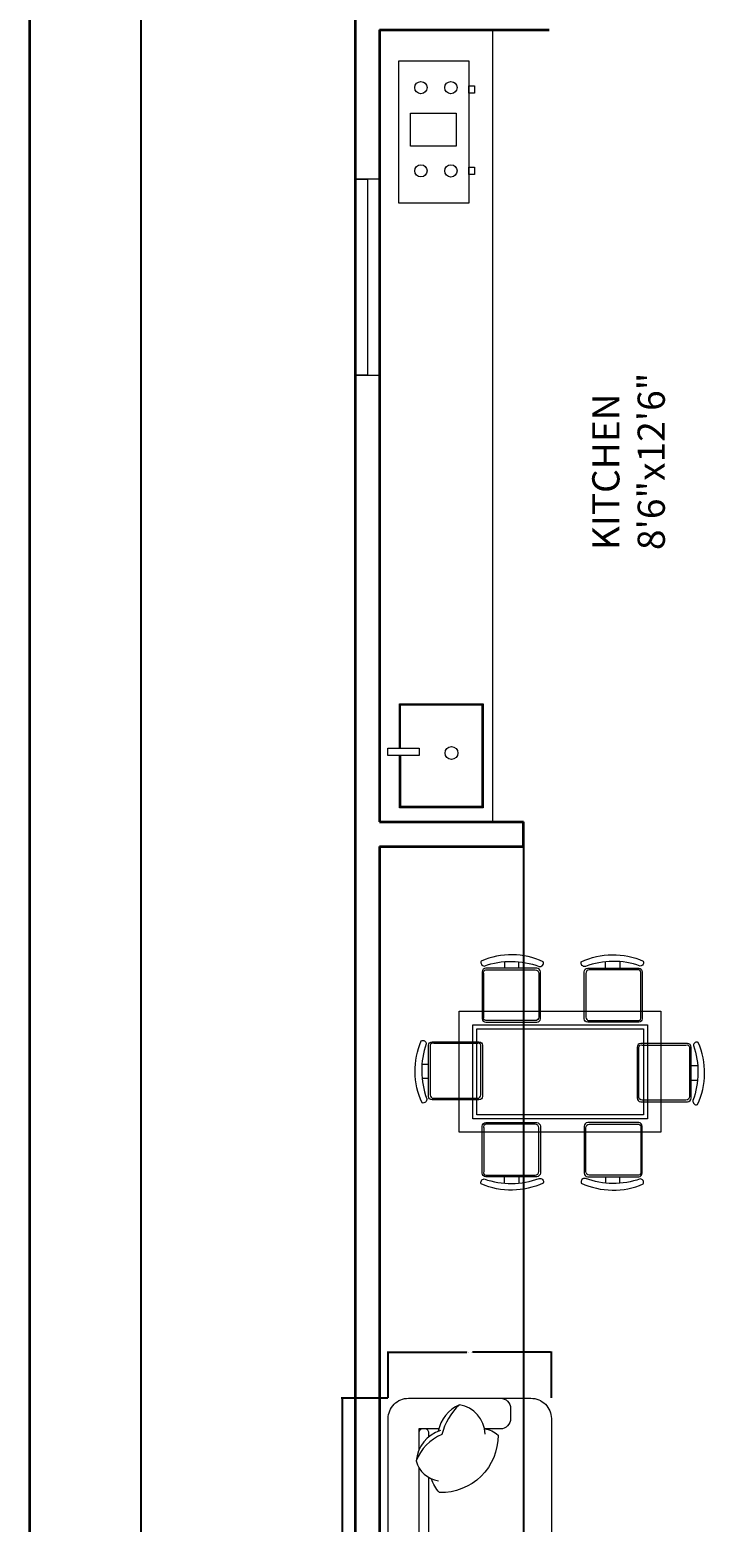
# Model space of a CAD drawing. Units: inches. Extents: x 1734 to 2405, y 1500 to 2491.
# Tile 11 of 14: x 1734 to 1862, y 2078 to 2352. Entities that reach past the tile are written whole.
import ezdxf

# ---------------------------------------------------------------- set-up
doc = ezdxf.new("R2010")
doc.units = ezdxf.units.IN
for name, color, linetype, lineweight in [('A-ANNO-DIMS', 2, 'Continuous', 18), ('A-ANNO-TTLB', 7, 'Continuous', 35), ('A-AREA-IDEN', 7, 'Continuous', 18), ('A-EQPM', 8, 'Continuous', 18), ('A-FLOR-CASE', 9, 'Continuous', 18), ('A-FLOR-FIXT', 9, 'Continuous', 18), ('A-FURN', 8, 'Continuous', 13), ('A-GLAZ', 4, 'Continuous', 18), ('A-WALL', 7, 'Continuous', 35)]:
    doc.layers.add(name, color=color, linetype=linetype, lineweight=lineweight)
doc.styles.get("Standard").update_dxf_attribs({"font": 'arial.ttf'})
doc.dimstyles.get("Standard").update_dxf_attribs({"dimtxt": 0.18, "dimasz": 0.18, "dimexe": 0.18, "dimexo": 0.0625, "dimgap": 0.09, "dimtad": 0, "dimtih": 1, "dimtoh": 1, "dimdec": 4, "dimzin": 0, "dimdsep": 46, "dimtxsty": 'Standard', "dimcen": 0.09, "dimadec": 0, "dimazin": 0, "dimtfac": 1, "dimtdec": 4, "dimtofl": 0, "dimtmove": 0, "dimatfit": 3, "dimfxl": 1, "dimtolj": 1, "dimtzin": 0, "dimarcsym": 0})

# ---------------------------------------------------------------- blocks, each defined once
blk = doc.blocks.new('SOFA-COMPACT')
at = {"ltscale": 0.03}
blk.add_lwpolyline([(29.99, 29.99, -0.414214), (28.12, 28.12, -0.414214), (29.99, 26.24), (29.99, 3.75, -0.414214), (26.24, 0), (3.75, 0, -0.414214), (0, 3.75), (0, 52.49, -0.414214), (3.75, 56.24), (26.24, 56.24, -0.414214), (29.99, 52.49), (29.99, 29.99, -0.414214), (28.12, 28.12, -0.414214), (29.99, 26.24)], format="xyb", dxfattribs=at)
for points in [[(13.1, 55.04, 0.14773), (9.88, 49.56, 0.213343), (5.16, 44.73, 0.178662)], [(17.83, 49.67, 0.356772), (13.1, 55.04, 0.249542), (9.21, 50.18, -9.61688)], [(20.62, 56.24, -0.414214), (22.49, 54.36), (22.49, 52.49, -0.414214), (20.62, 50.61), (17.72, 50.61)], [(9.63, 50.32, 0.306663), (5.16, 44.73, 0.30633), (9.24, 41.08, -0.872847)], [(7.5, 49.18), (7.5, 49.86, 0.414214), (6.75, 50.61), (6.37, 50.61, 0.414214), (5.62, 49.86)], [(5.62, 49.86), (5.62, 46.67, 0.414214)], [(17.71, 50.62, -0.165541), (20.19, 49.46, -0.425989), (9.45, 38.93, -0.121523), (7.97, 41.43, 7.115464)], [(5.62, 43.55), (5.62, 28.87, 0.414214), (6.37, 28.12), (6.75, 28.12, 0.414214), (7.5, 28.87), (7.5, 41.66, 0.414214)], [(5.62, 22.78), (5.62, 27.37, -0.414214), (6.37, 28.12), (6.75, 28.12, -0.414214), (7.5, 27.37), (7.5, 24.67, -0.414214)], [(7.5, 29.99, 0.414214), (9.37, 28.12)], [(7.5, 29.99, 0.414214), (9.37, 28.12), (28.12, 28.12, 0.414214)], [(7.5, 26.24, -0.414214), (9.37, 28.12)], [(7.5, 26.24, -0.414214), (9.37, 28.12), (28.12, 28.12, -0.414214)], [(9.63, 16.01, -0.306663), (5.16, 21.6, -0.30633), (9.24, 25.26, 0.872847)], [(17.71, 15.72, 0.165541), (20.19, 16.88, 0.425989), (9.45, 27.4, 0.121523), (7.97, 24.91, -7.115464)], [(13.1, 11.29, -0.14773), (9.88, 16.77, -0.213343), (5.16, 21.6, -0.178662)], [(5.62, 12.69), (5.62, 19.67, -0.414214)], [(7.5, 17.15), (7.5, 14.57, -0.414214)], [(17.83, 16.66, -0.356772), (13.1, 11.29, -0.249542), (9.21, 16.16, 9.61688)], [(9.63, 5.91, -0.306663), (5.16, 11.51, -0.30633), (9.24, 15.16, 0.872847)], [(8.71, 16.38, 0.071865), (7.97, 14.81, -7.115464)], [(17.71, 5.62, 0.165541), (20.19, 6.78, 0.200231), (17.17, 14.22, 0.121523)], [(13.1, 1.19, -0.14773), (9.88, 6.67, -0.213343), (5.16, 11.51, -0.178662)], [(5.62, 6.37), (5.62, 9.57, -0.414214)], [(5.62, 9.57), (5.62, 5.62), (9.31, 5.62, -0.414214)], [(7.5, 7.05), (7.5, 6.37, -0.414214), (6.75, 5.62), (6.37, 5.62, -0.414214), (5.62, 6.37)], [(17.83, 6.56, -0.356772), (13.1, 1.19, -0.249542), (9.21, 6.06, 9.61688)], [(17.72, 5.62), (20.62, 5.62, -0.414214), (22.49, 3.75), (22.49, 1.87, -0.414214), (20.62, 0)]]:
    blk.add_lwpolyline(points, format="xyb")
for points in [[(9.31, 50.61), (5.62, 50.61), (5.62, 46.67)], [(5.62, 43.55), (5.62, 22.78)], [(5.62, 19.67), (5.62, 12.69)]]:
    blk.add_lwpolyline(points)
blk.add_lwpolyline([(5.62, 28.87), (5.62, 27.37, -0.414214), (6.37, 28.12), (6.75, 28.12, -0.414214), (7.5, 27.37), (7.5, 28.87, -0.414214), (6.75, 28.12), (6.37, 28.12, -0.414214)], format="xyb", close=True)
blk = doc.blocks.new('*D12')
at = {"layer": 'A-ANNO-DIMS', "color": 0, "lineweight": -2, "transparency": 16777216}
for p, q in [((1799.89, 2100.96), (1791.34, 2100.96)), ((1791.52, 2100.78), (1791.52, 2073.03)), ((1791.52, 2044.91), (1791.52, 2072.66)), ((1799.89, 2044.73), (1791.34, 2044.73))]:
    blk.add_line(p, q, dxfattribs=at)
at = {"layer": 'A-ANNO-DIMS', "color": 0, "transparency": 16777216}
for points in [[(1791.49, 2100.78), (1791.55, 2100.78), (1791.52, 2100.96)], [(1791.49, 2044.91), (1791.55, 2044.91), (1791.52, 2044.73)]]:
    blk.add_solid(points, dxfattribs=at)
at = {"layer": 'Defpoints', "color": 0, "transparency": 16777216}
for p in [(1791.52, 2100.96), (1799.96, 2100.96), (1799.96, 2044.73)]:
    blk.add_point(p, dxfattribs=at)
at = {"layer": 'A-ANNO-DIMS', "color": 0, "transparency": 16777216, "insert": (1791.52, 2072.84), "char_height": 0.18, "attachment_point": 5}
blk.add_mtext('\\A1;SOFA 56 TYP.', dxfattribs=at)
blk = doc.blocks.new('*D13')
at = {"layer": 'A-ANNO-DIMS', "color": 0, "lineweight": -2, "transparency": 16777216}
for p, q in [((1799.96, 2101.02), (1799.96, 2109.58)), ((1800.14, 2109.4), (1814.42, 2109.4)), ((1829.77, 2109.4), (1815.48, 2109.4)), ((1829.95, 2101.02), (1829.95, 2109.58))]:
    blk.add_line(p, q, dxfattribs=at)
at = {"layer": 'A-ANNO-DIMS', "color": 0, "transparency": 16777216}
for points in [[(1800.14, 2109.43), (1800.14, 2109.37), (1799.96, 2109.4)], [(1829.77, 2109.43), (1829.77, 2109.37), (1829.95, 2109.4)]]:
    blk.add_solid(points, dxfattribs=at)
at = {"layer": 'Defpoints', "color": 0, "transparency": 16777216}
for p in [(1829.95, 2109.4), (1799.96, 2100.96), (1829.95, 2100.96)]:
    blk.add_point(p, dxfattribs=at)
at = {"layer": 'A-ANNO-DIMS', "color": 0, "transparency": 16777216, "insert": (1814.95, 2109.4), "char_height": 0.18, "attachment_point": 5}
blk.add_mtext('\\A1;30 TYP.', dxfattribs=at)
blk = doc.blocks.new('*D23')
at = {"layer": 'A-ANNO-DIMS', "color": 0, "lineweight": -2, "transparency": 16777216}
for p, q in [((1793.83, 2425.82), (1754.36, 2425.82)), ((1754.54, 2425.64), (1754.54, 2068.48)), ((1754.54, 1710.95), (1754.54, 2068.11)), ((1793.83, 1710.77), (1754.36, 1710.77))]:
    blk.add_line(p, q, dxfattribs=at)
at = {"layer": 'A-ANNO-DIMS', "color": 0, "transparency": 16777216}
for points in [[(1754.51, 2425.64), (1754.57, 2425.64), (1754.54, 2425.82)], [(1754.51, 1710.95), (1754.57, 1710.95), (1754.54, 1710.77)]]:
    blk.add_solid(points, dxfattribs=at)
at = {"layer": 'Defpoints', "color": 0, "transparency": 16777216}
for p in [(1754.54, 2425.82), (1793.89, 2425.82), (1793.89, 1710.77)]:
    blk.add_point(p, dxfattribs=at)
at = {"layer": 'A-ANNO-DIMS', "color": 0, "transparency": 16777216, "insert": (1754.54, 2068.3), "char_height": 0.18, "attachment_point": 5}
blk.add_mtext('\\A1;715', dxfattribs=at)
blk = doc.blocks.new('*D32')
at = {"layer": 'A-ANNO-DIMS', "color": 0, "lineweight": -2, "transparency": 16777216}
for p, q in [((1798.39, 2202.26), (1798.39, 1615.47)), ((1824.83, 2202.26), (1824.83, 1615.47)), ((1798.57, 1615.65), (1811.22, 1615.65)), ((1824.65, 1615.65), (1812.01, 1615.65))]:
    blk.add_line(p, q, dxfattribs=at)
at = {"layer": 'A-ANNO-DIMS', "color": 0, "transparency": 16777216}
for points in [[(1798.57, 1615.68), (1798.57, 1615.62), (1798.39, 1615.65)], [(1824.65, 1615.68), (1824.65, 1615.62), (1824.83, 1615.65)]]:
    blk.add_solid(points, dxfattribs=at)
at = {"layer": 'Defpoints', "color": 0, "transparency": 16777216}
for p in [(1798.39, 2202.32), (1824.83, 2202.32), (1824.83, 1615.65)]:
    blk.add_point(p, dxfattribs=at)
at = {"layer": 'A-ANNO-DIMS', "color": 0, "transparency": 16777216, "insert": (1811.61, 1615.65), "char_height": 0.18, "attachment_point": 5}
blk.add_mtext('\\A1;26.44', dxfattribs=at)
blk = doc.blocks.new('*D33')
at = {"layer": 'A-ANNO-DIMS', "color": 0, "lineweight": -2, "transparency": 16777216}
for p, q in [((1824.83, 2202.26), (1824.83, 1615.47)), ((1874.68, 2202.26), (1874.68, 1615.47)), ((1825.01, 1615.65), (1849.36, 1615.65)), ((1874.5, 1615.65), (1850.15, 1615.65))]:
    blk.add_line(p, q, dxfattribs=at)
at = {"layer": 'A-ANNO-DIMS', "color": 0, "transparency": 16777216}
for points in [[(1825.01, 1615.68), (1825.01, 1615.62), (1824.83, 1615.65)], [(1874.5, 1615.68), (1874.5, 1615.62), (1874.68, 1615.65)]]:
    blk.add_solid(points, dxfattribs=at)
at = {"layer": 'Defpoints', "color": 0, "transparency": 16777216}
for p in [(1824.83, 2202.32), (1874.68, 2202.32), (1874.68, 1615.65)]:
    blk.add_point(p, dxfattribs=at)
at = {"layer": 'A-ANNO-DIMS', "color": 0, "transparency": 16777216, "insert": (1849.76, 1615.65), "char_height": 0.18, "attachment_point": 5}
blk.add_mtext('\\A1;49.84', dxfattribs=at)

msp = doc.modelspace()

# ---------------------------------------------------------------- linework, layer by layer
at = {"layer": 'A-ANNO-TTLB'}
msp.add_lwpolyline([(1734.1307, 2491.1293), (2404.5589, 2491.1293), (2404.5589, 1500.293), (1734.1307, 1500.293)], close=True, dxfattribs=at)
at = {"layer": 'A-EQPM'}
for points in [[(1801.9497, 2346.6244), (1814.7817, 2346.6244), (1814.7817, 2320.5066), (1801.9497, 2320.5066)], [(1814.7817, 2342.041), (1815.82, 2342.041), (1815.82, 2340.6935), (1814.7817, 2340.6935)], [(1804.0877, 2336.9934), (1812.4457, 2336.9934), (1812.4457, 2330.9836), (1804.0877, 2330.9836)], [(1814.7817, 2327.0852), (1815.82, 2327.0852), (1815.82, 2325.7377), (1814.7817, 2325.7377)]]:
    msp.add_lwpolyline(points, close=True, dxfattribs=at)
for centre in [(1805.9861, 2341.7074), (1811.4968, 2341.7074), (1805.9861, 2326.4232), (1811.4968, 2326.4106)]:
    msp.add_circle(centre, 1.1254, dxfattribs=at)
at = {"layer": 'A-FLOR-CASE'}
msp.add_line((1819.2014, 2206.8246), (1819.2014, 2352.3246), dxfattribs=at)
at = {"layer": 'A-FLOR-FIXT'}
for p, q in [((1802.23, 2220.3738), (1802.23, 2228.5425)), ((1802.23, 2228.5425), (1802.23, 2228.4132)), ((1802.23, 2228.4132), (1802.23, 2228.3479)), ((1802.23, 2228.3479), (1817.4383, 2228.3479)), ((1817.4383, 2228.3479), (1817.1655, 2228.3479)), ((1817.1655, 2228.3479), (1817.1655, 2209.4249)), ((1802.0555, 2220.3738), (1802.23, 2220.3738)), ((1802.265, 2209.6534), (1802.265, 2219.0009)), ((1817.1655, 2209.6534), (1802.0555, 2209.6534)), ((1802.0555, 2209.6534), (1802.265, 2209.6534)), ((1817.1655, 2209.4249), (1817.1655, 2209.6534))]:
    msp.add_line(p, q, dxfattribs=at)
msp.add_lwpolyline([(1802.0555, 2220.3738), (1802.0555, 2228.5425), (1817.4383, 2228.5425), (1817.4383, 2209.4249), (1802.0555, 2209.4249), (1802.0555, 2219.0009)], dxfattribs=at)
msp.add_lwpolyline([(1799.9266, 2220.3738), (1805.6608, 2220.3738), (1805.6608, 2219.0009), (1799.9266, 2219.0009)], close=True, dxfattribs=at)
msp.add_circle((1811.5924, 2219.4842), 1.189, dxfattribs=at)
at = {"layer": 'A-FURN'}
for points in [[(1817.6044, 2180.3628, -0.17580919), (1827.6967, 2180.2863, 0.57839206), (1828.4613, 2181.127, 0.21452438), (1817.0692, 2181.2799, 0.55201397), (1817.6044, 2180.3628, -0.06507904)], [(1817.6044, 2180.3624, -0.17580919), (1827.6967, 2180.286, 0.57839206), (1828.4613, 2181.1267, 0.21452438), (1817.0692, 2181.2795, 0.55201397), (1817.6044, 2180.3624, -0.06507904)], [(1836.1931, 2180.2863, -0.57839206), (1835.4286, 2181.127, -0.21452438), (1846.8207, 2181.2799, -0.55201397), (1846.2855, 2180.3628, 0.1758092), (1836.1932, 2180.2863)], [(1836.1932, 2180.286, -0.57839206), (1835.4286, 2181.1267, -0.21452438), (1846.8207, 2181.2795, -0.55201397), (1846.2855, 2180.3624, 0.1758092), (1836.1932, 2180.286)], [(1827.2685, 2179.9577), (1817.8992, 2179.9577, 0.41421356), (1817.2437, 2179.3022), (1817.2437, 2170.6873, 0.41421356), (1817.8992, 2170.0318), (1827.2685, 2170.0318, 0.41421356), (1827.924, 2170.6873), (1827.924, 2179.3022, 0.41421356), (1827.2685, 2179.9577)], [(1827.2686, 2179.9573), (1817.8992, 2179.9573, 0.41421356), (1817.2437, 2179.3018), (1817.2437, 2170.6869, 0.41421356), (1817.8992, 2170.0314), (1827.2686, 2170.0314, 0.41421356), (1827.924, 2170.6869), (1827.924, 2179.3018, 0.41421356), (1827.2686, 2179.9573)], [(1823.9775, 2179.9577), (1823.9775, 2181.1427, -0.06475861)], [(1823.9776, 2179.9573), (1823.9776, 2181.1423, -0.06475861)], [(1845.9907, 2179.9577, -0.41421356), (1846.6462, 2179.3022), (1846.6462, 2170.6873, -0.41421356), (1845.9907, 2170.0318), (1836.6213, 2170.0318, -0.41421356), (1835.9658, 2170.6873), (1835.9658, 2179.3022, -0.41421356), (1836.6213, 2179.9577), (1845.9907, 2179.9577)], [(1845.9907, 2179.9573, -0.41421356), (1846.6462, 2179.3018), (1846.6462, 2170.6869, -0.41421356), (1845.9907, 2170.0314), (1836.6213, 2170.0314, -0.41421356), (1835.9658, 2170.6869), (1835.9658, 2179.3018, -0.41421356), (1836.6213, 2179.9573), (1845.9907, 2179.9573)], [(1839.9123, 2179.9577), (1839.9123, 2181.1427, 0.06475861)], [(1839.9123, 2179.9573), (1839.9123, 2181.1423, 0.06475861)], [(1807.0459, 2155.9913, -0.57839206), (1806.2052, 2155.2268, -0.21452438), (1806.0523, 2166.6189, -0.55201397), (1806.9694, 2166.0837, 0.17580937), (1807.0459, 2155.9913)], [(1807.0459, 2155.9909, -0.57839206), (1806.2052, 2155.2264, -0.21452438), (1806.0523, 2166.6185, -0.55201397), (1806.9695, 2166.0833, 0.17580937), (1807.0459, 2155.9909)], [(1807.3745, 2165.7889, -0.41421356), (1808.03, 2166.4444), (1816.645, 2166.4444, -0.41421356), (1817.3004, 2165.7889), (1817.3004, 2156.4195, -0.41421356), (1816.645, 2155.764), (1808.03, 2155.764, -0.41421356), (1807.3745, 2156.4195), (1807.3745, 2165.7889)], [(1807.3745, 2165.7885, -0.41421356), (1808.03, 2166.444), (1816.645, 2166.444, -0.41421356), (1817.3005, 2165.7885), (1817.3005, 2156.4191, -0.41421356), (1816.645, 2155.7636), (1808.03, 2155.7636, -0.41421356), (1807.3745, 2156.4191), (1807.3745, 2165.7885)], [(1855.6224, 2165.468, 0.41421356), (1854.9669, 2166.1235), (1846.3519, 2166.1235, 0.41421356), (1845.6965, 2165.468), (1845.6965, 2156.0986, 0.41421356), (1846.3519, 2155.4431), (1854.9669, 2155.4431, 0.41421356), (1855.6224, 2156.0986), (1855.6224, 2165.468)], [(1855.6224, 2165.4676, 0.41421356), (1854.9669, 2166.1231), (1846.352, 2166.1231, 0.41421356), (1845.6965, 2165.4676), (1845.6965, 2156.0982, 0.41421356), (1846.352, 2155.4427), (1854.9669, 2155.4427, 0.41421356), (1855.6224, 2156.0982), (1855.6224, 2165.4676)], [(1856.0275, 2165.7628, -0.17580919), (1855.951, 2155.6705, 0.57839206), (1856.7917, 2154.9059, 0.21452438), (1856.9446, 2166.298, 0.55201397), (1856.0275, 2165.7628, -0.06507904)], [(1856.0275, 2165.7624, -0.17580919), (1855.9511, 2155.6701, 0.57839206), (1856.7918, 2154.9055, 0.21452438), (1856.9446, 2166.2976, 0.55201397), (1856.0275, 2165.7624, -0.06507904)], [(1807.3745, 2159.7105), (1806.1896, 2159.7105, 0.06475861)], [(1807.3745, 2159.7101), (1806.1896, 2159.7101, 0.06475861)], [(1855.6224, 2159.3896), (1856.8073, 2159.3896, -0.06475861)], [(1855.6224, 2159.3892), (1856.8074, 2159.3892, -0.06475861)], [(1827.2685, 2141.6621), (1817.8992, 2141.6621, -0.41421356), (1817.2437, 2142.3176), (1817.2437, 2150.9326, -0.41421356), (1817.8992, 2151.5881), (1827.2685, 2151.5881, -0.41421356), (1827.924, 2150.9326), (1827.924, 2142.3176, -0.41421356), (1827.2685, 2141.6621)], [(1827.2686, 2141.6617), (1817.8992, 2141.6617, -0.41421356), (1817.2437, 2142.3172), (1817.2437, 2150.9322, -0.41421356), (1817.8992, 2151.5877), (1827.2686, 2151.5877, -0.41421356), (1827.924, 2150.9322), (1827.924, 2142.3172, -0.41421356), (1827.2686, 2141.6617)], [(1845.9907, 2141.6621, 0.41421356), (1846.6462, 2142.3176), (1846.6462, 2150.9326, 0.41421356), (1845.9907, 2151.5881), (1836.6213, 2151.5881, 0.41421356), (1835.9658, 2150.9326), (1835.9658, 2142.3176, 0.41421356), (1836.6213, 2141.6621), (1845.9907, 2141.6621)], [(1845.9907, 2141.6617, 0.41421356), (1846.6462, 2142.3172), (1846.6462, 2150.9322, 0.41421356), (1845.9907, 2151.5877), (1836.6213, 2151.5877, 0.41421356), (1835.9658, 2150.9322), (1835.9658, 2142.3172, 0.41421356), (1836.6213, 2141.6617), (1845.9907, 2141.6617)], [(1827.6967, 2141.3335, -0.57839206), (1828.4613, 2140.4928, -0.21452438), (1817.0692, 2140.3399, -0.55201397), (1817.6044, 2141.257, 0.17580929), (1827.6967, 2141.3335)], [(1827.6967, 2141.3331, -0.57839206), (1828.4613, 2140.4924, -0.21452438), (1817.0692, 2140.3395, -0.55201397), (1817.6044, 2141.2567, 0.17580929), (1827.6967, 2141.3331)], [(1823.9775, 2141.6621), (1823.9775, 2140.4772, 0.06475861)], [(1823.9776, 2141.6617), (1823.9776, 2140.4768, 0.06475861)], [(1846.2855, 2141.257, -0.17580928), (1836.1931, 2141.3335, 0.57839206), (1835.4286, 2140.4928, 0.21452438), (1846.8207, 2140.3399, 0.55201397), (1846.2855, 2141.257, -0.06507904)], [(1846.2855, 2141.2567, -0.17580928), (1836.1932, 2141.3331, 0.57839206), (1835.4286, 2140.4924, 0.21452438), (1846.8207, 2140.3395, 0.55201397), (1846.2855, 2141.2567, -0.06507904)], [(1839.9123, 2141.6621), (1839.9123, 2140.4772, -0.06475861)], [(1839.9123, 2141.6617), (1839.9123, 2140.4768, -0.06475861)]]:
    msp.add_lwpolyline(points, format="xyb", dxfattribs=at)
for points in [[(1817.9031, 2179.6624), (1826.9732, 2179.6624, -0.41421356), (1827.6287, 2179.0069), (1827.6287, 2170.9826, -0.41421356), (1826.9732, 2170.3271), (1817.9031, 2170.3271, -0.51206948), (1817.539, 2170.9826), (1817.539, 2179.0069, -0.51206948)], [(1817.9032, 2179.662), (1826.9732, 2179.662, -0.41421356), (1827.6287, 2179.0065), (1827.6287, 2170.9822, -0.41421356), (1826.9732, 2170.3267), (1817.9032, 2170.3267, -0.51206948), (1817.539, 2170.9822), (1817.539, 2179.0065, -0.51206948)], [(1845.9867, 2179.6624), (1836.9166, 2179.6624, 0.41421356), (1836.2611, 2179.0069), (1836.2611, 2170.9826, 0.41421356), (1836.9166, 2170.3271), (1845.9867, 2170.3271, 0.51206948), (1846.3509, 2170.9826), (1846.3509, 2179.0069, 0.51206948)], [(1845.9867, 2179.662), (1836.9166, 2179.662, 0.41421356), (1836.2612, 2179.0065), (1836.2612, 2170.9822, 0.41421356), (1836.9166, 2170.3267), (1845.9867, 2170.3267, 0.51206948), (1846.3509, 2170.9822), (1846.3509, 2179.0065, 0.51206948)], [(1807.6698, 2165.7849), (1807.6698, 2156.7148, 0.41421356), (1808.3253, 2156.0593), (1816.3497, 2156.0593, 0.41421356), (1817.0051, 2156.7148), (1817.0051, 2165.7849, 0.51206948), (1816.3497, 2166.1491), (1808.3253, 2166.1491, 0.51206948)], [(1807.6698, 2165.7845), (1807.6698, 2156.7144, 0.41421356), (1808.3253, 2156.0589), (1816.3497, 2156.0589, 0.41421356), (1817.0052, 2156.7144), (1817.0052, 2165.7845, 0.51206948), (1816.3497, 2166.1487), (1808.3253, 2166.1487, 0.51206948)], [(1855.3271, 2165.464), (1855.3271, 2156.3939, -0.41421356), (1854.6716, 2155.7384), (1846.6473, 2155.7384, -0.41421356), (1845.9918, 2156.3939), (1845.9918, 2165.464, -0.51206948), (1846.6473, 2165.8282), (1854.6716, 2165.8282, -0.51206948)], [(1855.3271, 2165.4636), (1855.3271, 2156.3935, -0.41421356), (1854.6716, 2155.738), (1846.6473, 2155.738, -0.41421356), (1845.9918, 2156.3935), (1845.9918, 2165.4636, -0.51206948), (1846.6473, 2165.8278), (1854.6716, 2165.8278, -0.51206948)], [(1817.9031, 2141.9574), (1826.9732, 2141.9574, 0.41421356), (1827.6287, 2142.6129), (1827.6287, 2150.6373, 0.41421356), (1826.9732, 2151.2927), (1817.9031, 2151.2927, 0.51206948), (1817.539, 2150.6373), (1817.539, 2142.6129, 0.51206948)], [(1817.9032, 2141.957), (1826.9732, 2141.957, 0.41421356), (1827.6287, 2142.6125), (1827.6287, 2150.6369, 0.41421356), (1826.9732, 2151.2924), (1817.9032, 2151.2924, 0.51206948), (1817.539, 2150.6369), (1817.539, 2142.6125, 0.51206948)], [(1845.9867, 2141.9574), (1836.9166, 2141.9574, -0.41421356), (1836.2611, 2142.6129), (1836.2611, 2150.6373, -0.41421356), (1836.9166, 2151.2927), (1845.9867, 2151.2927, -0.51206948), (1846.3509, 2150.6373), (1846.3509, 2142.6129, -0.51206948)], [(1845.9867, 2141.957), (1836.9166, 2141.957, -0.41421356), (1836.2612, 2142.6125), (1836.2612, 2150.6369, -0.41421356), (1836.9166, 2151.2924), (1845.9867, 2151.2924, -0.51206948), (1846.3509, 2150.6369), (1846.3509, 2142.6125, -0.51206948)]]:
    msp.add_lwpolyline(points, format="xyb", close=True, dxfattribs=at)
for points in [[(1821.3549, 2181.1642), (1821.3549, 2179.9577)], [(1821.3549, 2181.1638), (1821.3549, 2179.9573)], [(1842.5349, 2181.1642), (1842.5349, 2179.9577)], [(1842.535, 2181.1638), (1842.535, 2179.9573)], [(1806.168, 2162.3331), (1807.3745, 2162.3331)], [(1806.168, 2162.3327), (1807.3745, 2162.3327)], [(1856.8289, 2162.0122), (1855.6224, 2162.0122)], [(1856.8289, 2162.0119), (1855.6224, 2162.0119)], [(1821.3549, 2140.4556), (1821.3549, 2141.6621)], [(1821.3549, 2140.4552), (1821.3549, 2141.6617)], [(1842.5349, 2140.4556), (1842.5349, 2141.6621)], [(1842.535, 2140.4552), (1842.535, 2141.6617)]]:
    msp.add_lwpolyline(points, dxfattribs=at)
for points in [[(1813.0212, 2172.045), (1850.0748, 2172.045), (1850.0748, 2149.8129), (1813.0212, 2149.8129)], [(1813.0213, 2172.0446), (1850.0748, 2172.0446), (1850.0748, 2149.8125), (1813.0213, 2149.8125)], [(1815.4915, 2169.5748), (1847.6045, 2169.5748), (1847.6045, 2152.2832), (1815.4915, 2152.2832)], [(1815.4915, 2169.5744), (1847.6046, 2169.5744), (1847.6046, 2152.2828), (1815.4915, 2152.2828)], [(1816.2325, 2168.8337), (1846.8635, 2168.8337), (1846.8635, 2153.0242), (1816.2325, 2153.0242)], [(1816.2326, 2168.8333), (1846.8635, 2168.8333), (1846.8635, 2153.0238), (1816.2326, 2153.0238)]]:
    msp.add_lwpolyline(points, close=True, dxfattribs=at)
at = {"layer": 'A-GLAZ'}
for p, q in [((1798.3942, 2324.9064), (1793.8942, 2324.9064)), ((1793.8942, 2324.9064), (1796.1442, 2324.9064)), ((1796.1442, 2324.9064), (1796.1442, 2288.9064)), ((1796.1442, 2288.9064), (1793.8942, 2288.9064)), ((1793.8942, 2288.9064), (1798.3942, 2288.9064))]:
    msp.add_line(p, q, dxfattribs=at)
at = {"layer": 'A-WALL'}
for p, q in [((1793.8942, 2425.8246), (1793.8942, 1891.8246)), ((1798.3942, 2352.3246), (1829.5495, 2352.3246)), ((1798.3942, 2352.3246), (1798.3942, 2206.8246)), ((1798.3942, 2206.8246), (1824.8343, 2206.8246)), ((1824.8343, 2202.3246), (1824.8343, 2206.8246)), ((1798.3942, 2202.3246), (1824.8343, 2202.3246)), ((1798.3942, 2202.3246), (1798.3942, 1956.3246))]:
    msp.add_line(p, q, dxfattribs=at)

# ---------------------------------------------------------------- block references
at = {"layer": 'A-FURN'}
msp.add_blockref('SOFA-COMPACT', (1799.957, 2044.726), dxfattribs=at)

# ---------------------------------------------------------------- texts
at = {"layer": 'A-AREA-IDEN', "insert": (1837.4539, 2256.766), "char_height": 5, "attachment_point": 1, "rotation": 90}
msp.add_mtext_dynamic_manual_height_columns('KITCHEN\\P8\'6"x12\'6"', width=162.854422, gutter_width=12.5, heights=[0], dxfattribs=at)

# ---------------------------------------------------------------- dimensions: what is measured, and where the dimension line sits
at = {"layer": 'A-ANNO-DIMS'}
dim = msp.add_linear_dim(base=(1754.5442, 2425.8246), p1=(1793.8942, 1710.7667), p2=(1793.8942, 2425.8246), angle=90, dimstyle='Standard', override={"dimdec": 0, "dimlfac": 1, "dimrnd": 0, "dimzin": 0, "dimdsep": 46, "dimlunit": 2}, dxfattribs=at)
dim.commit()
dim.dimension.update_dxf_attribs({"geometry": '*D23', "text_midpoint": (1754.5442, 2068.2956)})
for base, p1, p2, picture, middle in [((1824.8343, 1615.6468), (1798.3942, 2202.3246), (1824.8343, 2202.3246), '*D32', (1811.6142, 1615.6468)), ((1874.676, 1615.6468), (1824.8343, 2202.3246), (1874.676, 2202.3246), '*D33', (1849.7551, 1615.6468))]:
    dim = msp.add_linear_dim(base=base, p1=p1, p2=p2, dimstyle='Standard', override={"dimdec": 2, "dimlfac": 1, "dimrnd": 0, "dimzin": 0, "dimdsep": 46, "dimlunit": 2}, dxfattribs=at)
    dim.commit()
    dim.dimension.update_dxf_attribs({"geometry": picture, "text_midpoint": middle})
dim = msp.add_linear_dim(base=(1829.9488, 2109.3966), p1=(1799.9567, 2100.9613), p2=(1829.9488, 2100.9613), text='<> TYP.', dimstyle='Standard', override={"dimdec": 0, "dimlfac": 1, "dimrnd": 0, "dimzin": 0, "dimdsep": 46, "dimlunit": 2}, dxfattribs=at)
dim.commit()
dim.dimension.update_dxf_attribs({"geometry": '*D13', "text_midpoint": (1814.9528, 2109.3966)})
dim = msp.add_linear_dim(base=(1791.5215, 2100.9613), p1=(1799.9567, 2044.7262), p2=(1799.9567, 2100.9613), angle=90, text='SOFA <> TYP.', dimstyle='Standard', override={"dimdec": 0, "dimlfac": 1, "dimrnd": 0, "dimzin": 0, "dimdsep": 46, "dimlunit": 2}, dxfattribs=at)
dim.commit()
dim.dimension.update_dxf_attribs({"geometry": '*D12', "text_midpoint": (1791.5215, 2072.8438)})

doc.saveas('drawing.dxf')
